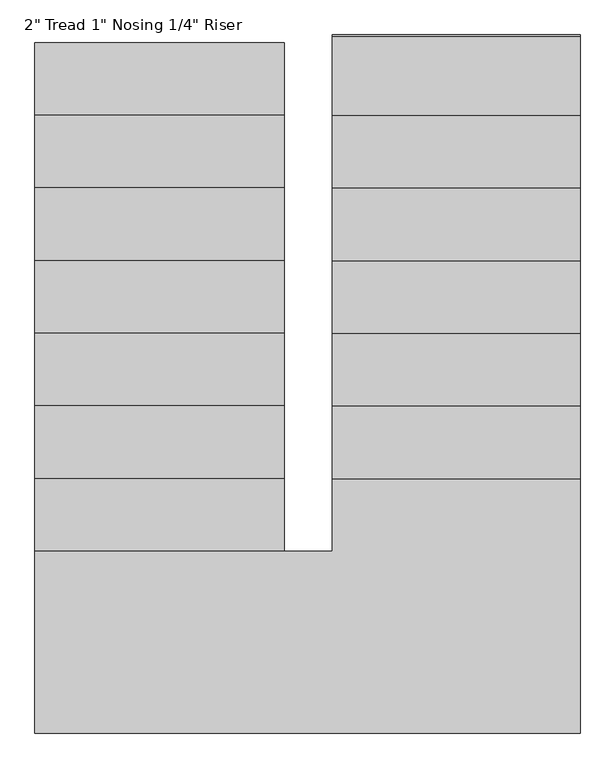
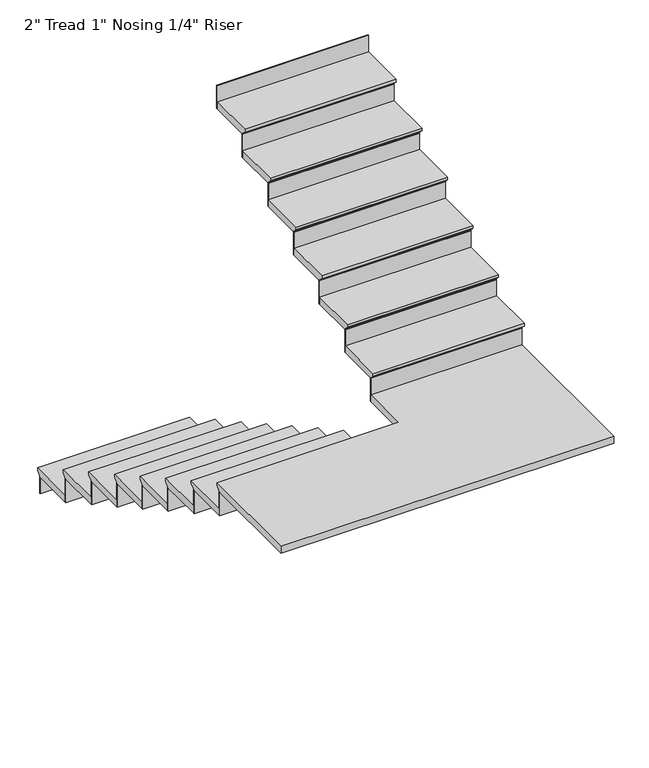
"""IFC4 building model written with IfcOpenShell, lengths in millimetres: stair flight geometry."""

from ifc_helpers import new_model, si_unit, origin, place, context, project, spatial, faceted_brep, source, transform, mapped, element, save


def stair_flight_c5737279(model_context):
    return source(origin(), model_context, "Body", "Brep", [
        faceted_brep([(-4232.280864, -3571.6080018, 19200.2833333), (-4232.280864, -3571.6080018, 19219.3333333), (-3187.6083919, -3571.6080018, 19219.3333333), (-3187.6083919, -3571.6080018, 19200.2833333), (-4232.280864, -3597.0080018, 19174.8833333), (-3187.6083919, -3597.0080018, 19174.8833333), (-4232.280864, -3901.8080018, 19219.3333333), (-3187.6083919, -3901.8080018, 19219.3333333), (-3187.6083919, -3597.0080018, 19168.5333333), (-3187.6083919, -3901.8080018, 19168.5333333), (-4232.280864, -3901.8080018, 19168.5333333), (-4232.280864, -3597.0080018, 19168.5333333)], [[[0, 1, 2, 3]], [[4, 0, 3, 5]], [[2, 1, 6, 7]], [[8, 9, 10, 11]], [[2, 7, 9, 8, 5, 3]], [[8, 11, 4, 5]], [[6, 1, 0, 4, 11, 10]], [[7, 6, 10, 9]]]),
        faceted_brep([(-4232.280864, -3597.0080018, 19168.5333333), (-4232.280864, -3597.0080018, 19050.0), (-4232.280864, -3603.3580018, 19050.0), (-4232.280864, -3603.3580018, 19168.5333333), (-3187.6083919, -3597.0080018, 19168.5333333), (-3187.6083919, -3603.3580018, 19168.5333333), (-3187.6083919, -3603.3580018, 19050.0), (-3187.6083919, -3597.0080018, 19050.0)], [[[0, 1, 2, 3]], [[4, 5, 6, 7]], [[1, 0, 4, 7]], [[2, 1, 7, 6]], [[3, 2, 6, 5]], [[0, 3, 5, 4]]]),
        faceted_brep([(-4232.280864, -3901.8080018, 19337.8666667), (-4232.280864, -3901.8080018, 19168.5333333), (-4232.280864, -3908.1580018, 19168.5333333), (-4232.280864, -3908.1580018, 19337.8666667), (-3187.6083919, -3901.8080018, 19337.8666667), (-3187.6083919, -3908.1580018, 19337.8666667), (-3187.6083919, -3908.1580018, 19168.5333333), (-3187.6083919, -3901.8080018, 19168.5333333)], [[[0, 1, 2, 3]], [[4, 5, 6, 7]], [[1, 0, 4, 7]], [[2, 1, 7, 6]], [[3, 2, 6, 5]], [[0, 3, 5, 4]]]),
        faceted_brep([(-3187.6083919, -3876.4080018, 19388.6666667), (-4232.280864, -3876.4080018, 19388.6666667), (-4232.280864, -4206.6080018, 19388.6666667), (-3187.6083919, -4206.6080018, 19388.6666667), (-3187.6083919, -3901.8080018, 19337.8666667), (-3187.6083919, -4206.6080018, 19337.8666667), (-4232.280864, -4206.6080018, 19337.8666667), (-4232.280864, -3901.8080018, 19337.8666667), (-3187.6083919, -3901.8080018, 19344.2166667), (-3187.6083919, -3876.4080018, 19369.6166667), (-4232.280864, -3901.8080018, 19344.2166667), (-4232.280864, -3876.4080018, 19369.6166667)], [[[0, 1, 2, 3]], [[4, 5, 6, 7]], [[0, 3, 5, 4, 8, 9]], [[4, 7, 10, 8]], [[2, 1, 11, 10, 7, 6]], [[3, 2, 6, 5]], [[11, 1, 0, 9]], [[10, 11, 9, 8]]]),
        faceted_brep([(-4232.280864, -4206.6080018, 19507.2), (-4232.280864, -4206.6080018, 19337.8666667), (-4232.280864, -4212.9580018, 19337.8666667), (-4232.280864, -4212.9580018, 19507.2), (-3187.6083919, -4206.6080018, 19507.2), (-3187.6083919, -4212.9580018, 19507.2), (-3187.6083919, -4212.9580018, 19337.8666667), (-3187.6083919, -4206.6080018, 19337.8666667)], [[[0, 1, 2, 3]], [[4, 5, 6, 7]], [[1, 0, 4, 7]], [[2, 1, 7, 6]], [[3, 2, 6, 5]], [[0, 3, 5, 4]]]),
        faceted_brep([(-3187.6083919, -4181.2080018, 19558.0), (-4232.280864, -4181.2080018, 19558.0), (-4232.280864, -4511.4080018, 19558.0), (-3187.6083919, -4511.4080018, 19558.0), (-3187.6083919, -4206.6080018, 19507.2), (-3187.6083919, -4511.4080018, 19507.2), (-4232.280864, -4511.4080018, 19507.2), (-4232.280864, -4206.6080018, 19507.2), (-3187.6083919, -4206.6080018, 19513.55), (-3187.6083919, -4181.2080018, 19538.95), (-4232.280864, -4206.6080018, 19513.55), (-4232.280864, -4181.2080018, 19538.95)], [[[0, 1, 2, 3]], [[4, 5, 6, 7]], [[0, 3, 5, 4, 8, 9]], [[4, 7, 10, 8]], [[2, 1, 11, 10, 7, 6]], [[3, 2, 6, 5]], [[11, 1, 0, 9]], [[10, 11, 9, 8]]]),
        faceted_brep([(-4232.280864, -4511.4080018, 19676.5333333), (-4232.280864, -4511.4080018, 19507.2), (-4232.280864, -4517.7580018, 19507.2), (-4232.280864, -4517.7580018, 19676.5333333), (-3187.6083919, -4511.4080018, 19676.5333333), (-3187.6083919, -4517.7580018, 19676.5333333), (-3187.6083919, -4517.7580018, 19507.2), (-3187.6083919, -4511.4080018, 19507.2)], [[[0, 1, 2, 3]], [[4, 5, 6, 7]], [[1, 0, 4, 7]], [[2, 1, 7, 6]], [[3, 2, 6, 5]], [[0, 3, 5, 4]]]),
        faceted_brep([(-3187.6083919, -4486.0080018, 19727.3333333), (-4232.280864, -4486.0080018, 19727.3333333), (-4232.280864, -4816.2080018, 19727.3333333), (-3187.6083919, -4816.2080018, 19727.3333333), (-3187.6083919, -4511.4080018, 19676.5333333), (-3187.6083919, -4816.2080018, 19676.5333333), (-4232.280864, -4816.2080018, 19676.5333333), (-4232.280864, -4511.4080018, 19676.5333333), (-3187.6083919, -4511.4080018, 19682.8833333), (-3187.6083919, -4486.0080018, 19708.2833333), (-4232.280864, -4511.4080018, 19682.8833333), (-4232.280864, -4486.0080018, 19708.2833333)], [[[0, 1, 2, 3]], [[4, 5, 6, 7]], [[0, 3, 5, 4, 8, 9]], [[4, 7, 10, 8]], [[2, 1, 11, 10, 7, 6]], [[3, 2, 6, 5]], [[11, 1, 0, 9]], [[10, 11, 9, 8]]]),
        faceted_brep([(-4232.280864, -4816.2080018, 19845.8666667), (-4232.280864, -4816.2080018, 19676.5333333), (-4232.280864, -4822.5580018, 19676.5333333), (-4232.280864, -4822.5580018, 19845.8666667), (-3187.6083919, -4816.2080018, 19845.8666667), (-3187.6083919, -4822.5580018, 19845.8666667), (-3187.6083919, -4822.5580018, 19676.5333333), (-3187.6083919, -4816.2080018, 19676.5333333)], [[[0, 1, 2, 3]], [[4, 5, 6, 7]], [[1, 0, 4, 7]], [[2, 1, 7, 6]], [[3, 2, 6, 5]], [[0, 3, 5, 4]]]),
        faceted_brep([(-3187.6083919, -4790.8080018, 19896.6666667), (-4232.280864, -4790.8080018, 19896.6666667), (-4232.280864, -5121.0080018, 19896.6666667), (-3187.6083919, -5121.0080018, 19896.6666667), (-3187.6083919, -4816.2080018, 19845.8666667), (-3187.6083919, -5121.0080018, 19845.8666667), (-4232.280864, -5121.0080018, 19845.8666667), (-4232.280864, -4816.2080018, 19845.8666667), (-3187.6083919, -4816.2080018, 19852.2166667), (-3187.6083919, -4790.8080018, 19877.6166667), (-4232.280864, -4816.2080018, 19852.2166667), (-4232.280864, -4790.8080018, 19877.6166667)], [[[0, 1, 2, 3]], [[4, 5, 6, 7]], [[0, 3, 5, 4, 8, 9]], [[4, 7, 10, 8]], [[2, 1, 11, 10, 7, 6]], [[3, 2, 6, 5]], [[11, 1, 0, 9]], [[10, 11, 9, 8]]]),
        faceted_brep([(-4232.280864, -5121.0080018, 20015.2), (-4232.280864, -5121.0080018, 19845.8666667), (-4232.280864, -5127.3580018, 19845.8666667), (-4232.280864, -5127.3580018, 20015.2), (-3187.6083919, -5121.0080018, 20015.2), (-3187.6083919, -5127.3580018, 20015.2), (-3187.6083919, -5127.3580018, 19845.8666667), (-3187.6083919, -5121.0080018, 19845.8666667)], [[[0, 1, 2, 3]], [[4, 5, 6, 7]], [[1, 0, 4, 7]], [[2, 1, 7, 6]], [[3, 2, 6, 5]], [[0, 3, 5, 4]]]),
        faceted_brep([(-3187.6083919, -5095.6080018, 20066.0), (-4232.280864, -5095.6080018, 20066.0), (-4232.280864, -5425.8080018, 20066.0), (-3187.6083919, -5425.8080018, 20066.0), (-3187.6083919, -5121.0080018, 20015.2), (-3187.6083919, -5425.8080018, 20015.2), (-4232.280864, -5425.8080018, 20015.2), (-4232.280864, -5121.0080018, 20015.2), (-3187.6083919, -5121.0080018, 20021.55), (-3187.6083919, -5095.6080018, 20046.95), (-4232.280864, -5121.0080018, 20021.55), (-4232.280864, -5095.6080018, 20046.95)], [[[0, 1, 2, 3]], [[4, 5, 6, 7]], [[0, 3, 5, 4, 8, 9]], [[4, 7, 10, 8]], [[2, 1, 11, 10, 7, 6]], [[3, 2, 6, 5]], [[11, 1, 0, 9]], [[10, 11, 9, 8]]]),
        faceted_brep([(-4232.280864, -5425.8080018, 20184.5333333), (-4232.280864, -5425.8080018, 20015.2), (-4232.280864, -5432.1580018, 20015.2), (-4232.280864, -5432.1580018, 20184.5333333), (-3187.6083919, -5425.8080018, 20184.5333333), (-3187.6083919, -5432.1580018, 20184.5333333), (-3187.6083919, -5432.1580018, 20015.2), (-3187.6083919, -5425.8080018, 20015.2)], [[[0, 1, 2, 3]], [[4, 5, 6, 7]], [[1, 0, 4, 7]], [[2, 1, 7, 6]], [[3, 2, 6, 5]], [[0, 3, 5, 4]]]),
        faceted_brep([(-3187.6083919, -5400.4080018, 20235.3333333), (-4232.280864, -5400.4080018, 20235.3333333), (-4232.280864, -5730.6080018, 20235.3333333), (-3187.6083919, -5730.6080018, 20235.3333333), (-3187.6083919, -5425.8080018, 20184.5333333), (-3187.6083919, -5730.6080018, 20184.5333333), (-4232.280864, -5730.6080018, 20184.5333333), (-4232.280864, -5425.8080018, 20184.5333333), (-3187.6083919, -5425.8080018, 20190.8833333), (-3187.6083919, -5400.4080018, 20216.2833333), (-4232.280864, -5425.8080018, 20190.8833333), (-4232.280864, -5400.4080018, 20216.2833333)], [[[0, 1, 2, 3]], [[4, 5, 6, 7]], [[0, 3, 5, 4, 8, 9]], [[4, 7, 10, 8]], [[2, 1, 11, 10, 7, 6]], [[3, 2, 6, 5]], [[11, 1, 0, 9]], [[10, 11, 9, 8]]]),
        faceted_brep([(-4232.280864, -5730.6080018, 20353.8666667), (-4232.280864, -5730.6080018, 20184.5333333), (-4232.280864, -5736.9580018, 20184.5333333), (-4232.280864, -5736.9580018, 20353.8666667), (-3187.6083919, -5730.6080018, 20353.8666667), (-3187.6083919, -5736.9580018, 20353.8666667), (-3187.6083919, -5736.9580018, 20184.5333333), (-3187.6083919, -5730.6080018, 20184.5333333)], [[[0, 1, 2, 3]], [[4, 5, 6, 7]], [[1, 0, 4, 7]], [[2, 1, 7, 6]], [[3, 2, 6, 5]], [[0, 3, 5, 4]]]),
        faceted_brep([(-2984.4083919, -5375.0080018, 20404.6666667), (-2984.4083919, -5705.2080018, 20404.6666667), (-4232.280864, -5705.2080018, 20404.6666667), (-4232.280864, -6467.2080018, 20404.6666667), (-1946.280864, -6467.2080018, 20404.6666667), (-1946.280864, -5375.0080018, 20404.6666667), (-2984.4083919, -5705.2080018, 20353.8666667), (-2984.4083919, -5375.0080018, 20353.8666667), (-1946.280864, -5375.0080018, 20353.8666667), (-1946.280864, -6467.2080018, 20353.8666667), (-4232.280864, -6467.2080018, 20353.8666667), (-4232.280864, -5730.6080018, 20353.8666667), (-3187.6083919, -5730.6080018, 20353.8666667), (-3187.6083919, -5705.2080018, 20353.8666667), (-3187.6083919, -5705.2080018, 20385.6166667), (-4232.280864, -5705.2080018, 20385.6166667), (-3187.6083919, -5730.6080018, 20360.2166667), (-4232.280864, -5730.6080018, 20360.2166667)], [[[0, 1, 2, 3, 4, 5]], [[6, 7, 8, 9, 10, 11, 12, 13]], [[1, 0, 7, 6]], [[2, 1, 6, 13, 14, 15]], [[13, 12, 16, 14]], [[12, 11, 17, 16]], [[3, 2, 15, 17, 11, 10]], [[4, 3, 10, 9]], [[5, 4, 9, 8]], [[0, 5, 8, 7]], [[17, 15, 14, 16]]]),
        faceted_brep([(-1946.280864, -5375.0080018, 20523.2), (-1946.280864, -5375.0080018, 20353.8666667), (-1946.280864, -5368.6580018, 20353.8666667), (-1946.280864, -5368.6580018, 20523.2), (-2984.4083919, -5375.0080018, 20523.2), (-2984.4083919, -5368.6580018, 20523.2), (-2984.4083919, -5368.6580018, 20353.8666667), (-2984.4083919, -5375.0080018, 20353.8666667)], [[[0, 1, 2, 3]], [[4, 5, 6, 7]], [[1, 0, 4, 7]], [[2, 1, 7, 6]], [[3, 2, 6, 5]], [[0, 3, 5, 4]]]),
        faceted_brep([(-2984.4083919, -5400.4080018, 20574.0), (-1946.280864, -5400.4080018, 20574.0), (-1946.280864, -5070.2080018, 20574.0), (-2984.4083919, -5070.2080018, 20574.0), (-2984.4083919, -5375.0080018, 20523.2), (-2984.4083919, -5070.2080018, 20523.2), (-1946.280864, -5070.2080018, 20523.2), (-1946.280864, -5375.0080018, 20523.2), (-2984.4083919, -5375.0080018, 20529.55), (-2984.4083919, -5400.4080018, 20554.95), (-1946.280864, -5375.0080018, 20529.55), (-1946.280864, -5400.4080018, 20554.95)], [[[0, 1, 2, 3]], [[4, 5, 6, 7]], [[0, 3, 5, 4, 8, 9]], [[4, 7, 10, 8]], [[2, 1, 11, 10, 7, 6]], [[3, 2, 6, 5]], [[11, 1, 0, 9]], [[10, 11, 9, 8]]]),
        faceted_brep([(-1946.280864, -5070.2080018, 20692.5333333), (-1946.280864, -5070.2080018, 20523.2), (-1946.280864, -5063.8580018, 20523.2), (-1946.280864, -5063.8580018, 20692.5333333), (-2984.4083919, -5070.2080018, 20692.5333333), (-2984.4083919, -5063.8580018, 20692.5333333), (-2984.4083919, -5063.8580018, 20523.2), (-2984.4083919, -5070.2080018, 20523.2)], [[[0, 1, 2, 3]], [[4, 5, 6, 7]], [[1, 0, 4, 7]], [[2, 1, 7, 6]], [[3, 2, 6, 5]], [[0, 3, 5, 4]]]),
        faceted_brep([(-2984.4083919, -5095.6080018, 20743.3333333), (-1946.280864, -5095.6080018, 20743.3333333), (-1946.280864, -4765.4080018, 20743.3333333), (-2984.4083919, -4765.4080018, 20743.3333333), (-2984.4083919, -5070.2080018, 20692.5333333), (-2984.4083919, -4765.4080018, 20692.5333333), (-1946.280864, -4765.4080018, 20692.5333333), (-1946.280864, -5070.2080018, 20692.5333333), (-2984.4083919, -5070.2080018, 20698.8833333), (-2984.4083919, -5095.6080018, 20724.2833333), (-1946.280864, -5070.2080018, 20698.8833333), (-1946.280864, -5095.6080018, 20724.2833333)], [[[0, 1, 2, 3]], [[4, 5, 6, 7]], [[0, 3, 5, 4, 8, 9]], [[4, 7, 10, 8]], [[2, 1, 11, 10, 7, 6]], [[3, 2, 6, 5]], [[11, 1, 0, 9]], [[10, 11, 9, 8]]]),
        faceted_brep([(-1946.280864, -4765.4080018, 20861.8666667), (-1946.280864, -4765.4080018, 20692.5333333), (-1946.280864, -4759.0580018, 20692.5333333), (-1946.280864, -4759.0580018, 20861.8666667), (-2984.4083919, -4765.4080018, 20861.8666667), (-2984.4083919, -4759.0580018, 20861.8666667), (-2984.4083919, -4759.0580018, 20692.5333333), (-2984.4083919, -4765.4080018, 20692.5333333)], [[[0, 1, 2, 3]], [[4, 5, 6, 7]], [[1, 0, 4, 7]], [[2, 1, 7, 6]], [[3, 2, 6, 5]], [[0, 3, 5, 4]]]),
        faceted_brep([(-2984.4083919, -4790.8080018, 20912.6666667), (-1946.280864, -4790.8080018, 20912.6666667), (-1946.280864, -4460.6080018, 20912.6666667), (-2984.4083919, -4460.6080018, 20912.6666667), (-2984.4083919, -4765.4080018, 20861.8666667), (-2984.4083919, -4460.6080018, 20861.8666667), (-1946.280864, -4460.6080018, 20861.8666667), (-1946.280864, -4765.4080018, 20861.8666667), (-2984.4083919, -4765.4080018, 20868.2166667), (-2984.4083919, -4790.8080018, 20893.6166667), (-1946.280864, -4765.4080018, 20868.2166667), (-1946.280864, -4790.8080018, 20893.6166667)], [[[0, 1, 2, 3]], [[4, 5, 6, 7]], [[0, 3, 5, 4, 8, 9]], [[4, 7, 10, 8]], [[2, 1, 11, 10, 7, 6]], [[3, 2, 6, 5]], [[11, 1, 0, 9]], [[10, 11, 9, 8]]]),
        faceted_brep([(-1946.280864, -4460.6080018, 21031.2), (-1946.280864, -4460.6080018, 20861.8666667), (-1946.280864, -4454.2580018, 20861.8666667), (-1946.280864, -4454.2580018, 21031.2), (-2984.4083919, -4460.6080018, 21031.2), (-2984.4083919, -4454.2580018, 21031.2), (-2984.4083919, -4454.2580018, 20861.8666667), (-2984.4083919, -4460.6080018, 20861.8666667)], [[[0, 1, 2, 3]], [[4, 5, 6, 7]], [[1, 0, 4, 7]], [[2, 1, 7, 6]], [[3, 2, 6, 5]], [[0, 3, 5, 4]]]),
        faceted_brep([(-2984.4083919, -4486.0080018, 21082.0), (-1946.280864, -4486.0080018, 21082.0), (-1946.280864, -4155.8080018, 21082.0), (-2984.4083919, -4155.8080018, 21082.0), (-2984.4083919, -4460.6080018, 21031.2), (-2984.4083919, -4155.8080018, 21031.2), (-1946.280864, -4155.8080018, 21031.2), (-1946.280864, -4460.6080018, 21031.2), (-2984.4083919, -4460.6080018, 21037.55), (-2984.4083919, -4486.0080018, 21062.95), (-1946.280864, -4460.6080018, 21037.55), (-1946.280864, -4486.0080018, 21062.95)], [[[0, 1, 2, 3]], [[4, 5, 6, 7]], [[0, 3, 5, 4, 8, 9]], [[4, 7, 10, 8]], [[2, 1, 11, 10, 7, 6]], [[3, 2, 6, 5]], [[11, 1, 0, 9]], [[10, 11, 9, 8]]]),
        faceted_brep([(-1946.280864, -4155.8080018, 21200.5333333), (-1946.280864, -4155.8080018, 21031.2), (-1946.280864, -4149.4580018, 21031.2), (-1946.280864, -4149.4580018, 21200.5333333), (-2984.4083919, -4155.8080018, 21200.5333333), (-2984.4083919, -4149.4580018, 21200.5333333), (-2984.4083919, -4149.4580018, 21031.2), (-2984.4083919, -4155.8080018, 21031.2)], [[[0, 1, 2, 3]], [[4, 5, 6, 7]], [[1, 0, 4, 7]], [[2, 1, 7, 6]], [[3, 2, 6, 5]], [[0, 3, 5, 4]]]),
        faceted_brep([(-2984.4083919, -4181.2080018, 21251.3333333), (-1946.280864, -4181.2080018, 21251.3333333), (-1946.280864, -3851.0080018, 21251.3333333), (-2984.4083919, -3851.0080018, 21251.3333333), (-2984.4083919, -4155.8080018, 21200.5333333), (-2984.4083919, -3851.0080018, 21200.5333333), (-1946.280864, -3851.0080018, 21200.5333333), (-1946.280864, -4155.8080018, 21200.5333333), (-2984.4083919, -4155.8080018, 21206.8833333), (-2984.4083919, -4181.2080018, 21232.2833333), (-1946.280864, -4155.8080018, 21206.8833333), (-1946.280864, -4181.2080018, 21232.2833333)], [[[0, 1, 2, 3]], [[4, 5, 6, 7]], [[0, 3, 5, 4, 8, 9]], [[4, 7, 10, 8]], [[2, 1, 11, 10, 7, 6]], [[3, 2, 6, 5]], [[11, 1, 0, 9]], [[10, 11, 9, 8]]]),
        faceted_brep([(-1946.280864, -3851.0080018, 21369.8666667), (-1946.280864, -3851.0080018, 21200.5333333), (-1946.280864, -3844.6580018, 21200.5333333), (-1946.280864, -3844.6580018, 21369.8666667), (-2984.4083919, -3851.0080018, 21369.8666667), (-2984.4083919, -3844.6580018, 21369.8666667), (-2984.4083919, -3844.6580018, 21200.5333333), (-2984.4083919, -3851.0080018, 21200.5333333)], [[[0, 1, 2, 3]], [[4, 5, 6, 7]], [[1, 0, 4, 7]], [[2, 1, 7, 6]], [[3, 2, 6, 5]], [[0, 3, 5, 4]]]),
        faceted_brep([(-1946.280864, -3546.2080018, 21539.2), (-1946.280864, -3546.2080018, 21369.8666667), (-1946.280864, -3539.8580018, 21369.8666667), (-1946.280864, -3539.8580018, 21539.2), (-2984.4083919, -3546.2080018, 21539.2), (-2984.4083919, -3539.8580018, 21539.2), (-2984.4083919, -3539.8580018, 21369.8666667), (-2984.4083919, -3546.2080018, 21369.8666667)], [[[0, 1, 2, 3]], [[4, 5, 6, 7]], [[1, 0, 4, 7]], [[2, 1, 7, 6]], [[3, 2, 6, 5]], [[0, 3, 5, 4]]]),
        faceted_brep([(-2984.4083919, -3876.4080018, 21420.6666667), (-1946.280864, -3876.4080018, 21420.6666667), (-1946.280864, -3546.2080018, 21420.6666667), (-2984.4083919, -3546.2080018, 21420.6666667), (-2984.4083919, -3851.0080018, 21369.8666667), (-2984.4083919, -3546.2080018, 21369.8666667), (-1946.280864, -3546.2080018, 21369.8666667), (-1946.280864, -3851.0080018, 21369.8666667), (-2984.4083919, -3851.0080018, 21376.2166667), (-2984.4083919, -3876.4080018, 21401.6166667), (-1946.280864, -3851.0080018, 21376.2166667), (-1946.280864, -3876.4080018, 21401.6166667)], [[[0, 1, 2, 3]], [[4, 5, 6, 7]], [[0, 3, 5, 4, 8, 9]], [[4, 7, 10, 8]], [[2, 1, 11, 10, 7, 6]], [[3, 2, 6, 5]], [[11, 1, 0, 9]], [[10, 11, 9, 8]]]),
    ])


if __name__ == "__main__":
    model = new_model("IFC4")
    model_context = context("Model", 3, world=origin())
    ifc_project = project(units=[si_unit("LENGTHUNIT", "METRE", prefix="MILLI")], contexts=[model_context])
    site = spatial("IfcSite", under=ifc_project)
    building = spatial("IfcBuilding", under=site)
    placement = place(None, origin())
    stair_flight_shape = stair_flight_c5737279(model_context)
    element("IfcStairFlight", 1, ObjectType="2\" Tread 1\" Nosing 1/4\" Riser", at=placement, inside=building, context=model_context, shape_type="MappedRepresentation", body=[
        mapped(stair_flight_shape, transform((0.0, 0.0, 0.0), x_axis=(1.0, 0.0, 0.0), y_axis=(0.0, 1.0, 0.0), z_axis=(0.0, 0.0, 1.0))),
    ])
    save(model, "model.ifc")
